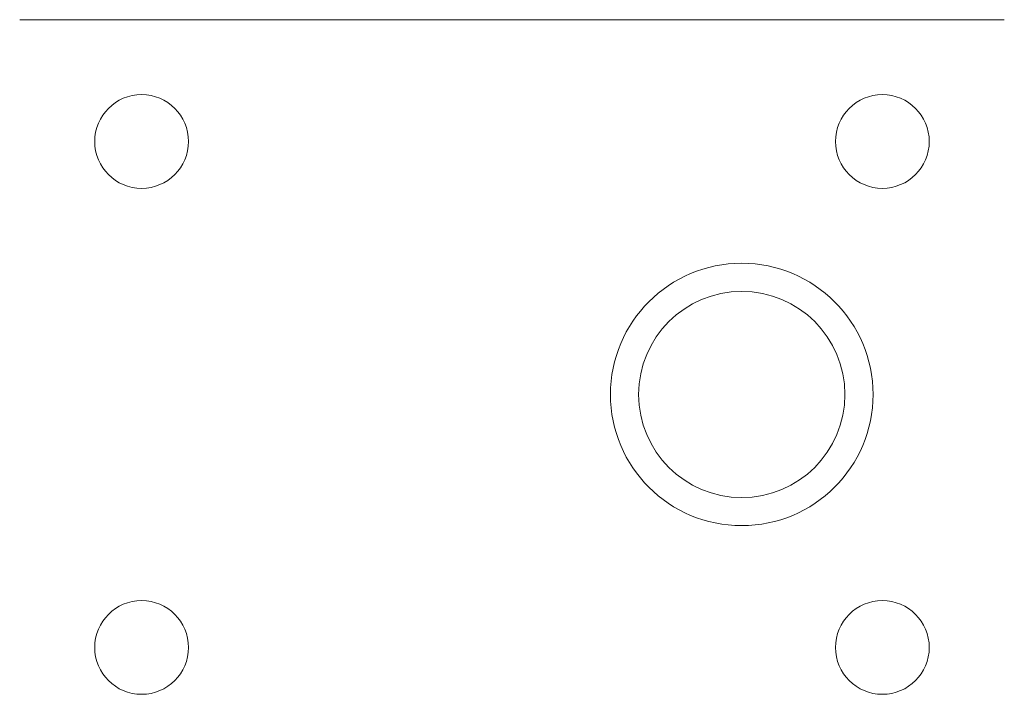
# Model space of a CAD drawing. Units: millimetres. Extents: x 173 to 278, y -72 to 0.
import ezdxf

# ---------------------------------------------------------------- set-up
doc = ezdxf.new("R2010")
doc.units = ezdxf.units.MM
doc.layers.add('M-CONS', color=8, linetype='Continuous', lineweight=18)

msp = doc.modelspace()

# ---------------------------------------------------------------- linework, layer by layer
at = {"layer": 'M-CONS', "extrusion": (0, -1, 0)}
msp.add_lwpolyline([(187.83, -8.05), (267.83, -8.05), (267.83, -14.05), (277.83, -14.05), (277.83, -0.05), (249.83, -0.05), (249.83, 18.95, 1), (205.83, 18.95), (205.83, -0.05), (172.83, -0.05), (172.83, -14.05), (182.83, -14.05), (182.83, -8.05), (227.83, -8.05)], format="xyb", dxfattribs=at)
msp.add_circle((227.83, 18.95), 16, dxfattribs=at)
at = {"layer": 'M-CONS'}
for centre, radius in [((185.83, -13, -0.05), 5), ((264.83, -13, -0.05), 5), ((249.83, -40, -0.05), 14), ((249.83, -40, -0.05), 11), ((185.83, -67, -0.05), 5), ((264.83, -67, -0.05), 5)]:
    msp.add_circle(centre, radius, dxfattribs=at)

doc.saveas('drawing.dxf')
